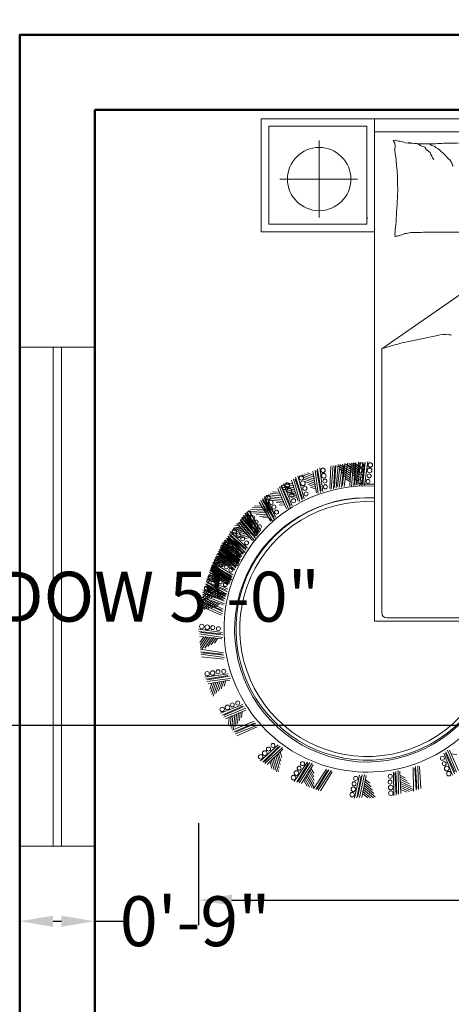
# Model space of a CAD drawing. Units: inches. Extents: x -59 to 502, y -260 to 136.
# Tile 3 of 8: x 25 to 77, y -53 to 66. Entities that reach past the tile are written whole.
import ezdxf

# ---------------------------------------------------------------- set-up
doc = ezdxf.new("R2010")
doc.units = ezdxf.units.IN
doc.header["$MEASUREMENT"] = 0
for name, color, linetype, lineweight in [('A-ANNO-DIMS', 2, 'Continuous', 18), ('Beds', 122, 'Continuous', 18), ('Outer Wall', 10, 'Continuous', 50), ('Windows', 150, 'Continuous', 18)]:
    doc.layers.add(name, color=color, linetype=linetype, lineweight=lineweight)
doc.styles.add('DIM_FONT', font='SIMPLEX.shx', dxfattribs={"width": 0.8})
doc.styles.get("Standard").update_dxf_attribs({"font": 'arial.ttf'})
doc.dimstyles.get("Standard").update_dxf_attribs({"dimtxt": 6, "dimasz": 4, "dimexe": 3, "dimexo": 3, "dimgap": 0.09, "dimtad": 0, "dimtih": 1, "dimtoh": 1, "dimdec": 1, "dimzin": 0, "dimdsep": 46, "dimlunit": 3, "dimtxsty": 'Standard', "dimcen": 0.09, "dimadec": 0, "dimazin": 0, "dimtfac": 1, "dimtdec": 1, "dimtofl": 0, "dimtmove": 0, "dimatfit": 3, "dimfxl": 1, "dimtolj": 1, "dimtzin": 0, "dimarcsym": 0})

# ---------------------------------------------------------------- blocks, each defined once
blk = doc.blocks.new('*D6')
at = {"layer": 'A-ANNO-DIMS', "color": 0, "lineweight": -2, "transparency": 16777216}
for p, q in [((22.46, 63.92), (-2.69, 63.92)), ((0.31, 59.92), (0.31, -58.98)), ((0.31, -184.08), (0.31, -65.18)), ((22.46, -188.08), (-2.69, -188.08))]:
    blk.add_line(p, q, dxfattribs=at)
at = {"layer": 'A-ANNO-DIMS', "color": 0, "transparency": 16777216}
for points in [[(-0.35, 59.92), (0.98, 59.92), (0.31, 63.92)], [(-0.35, -184.08), (0.98, -184.08), (0.31, -188.08)]]:
    blk.add_solid(points, dxfattribs=at)
at = {"layer": 'Defpoints', "color": 0, "transparency": 16777216}
for p in [(25.46, 63.92), (0.31, -188.08), (25.46, -188.08)]:
    blk.add_point(p, dxfattribs=at)
at = {"layer": 'A-ANNO-DIMS', "color": 0, "transparency": 16777216, "insert": (0.31, -62.08), "char_height": 6, "attachment_point": 5}
blk.add_mtext("\\A1;21'", dxfattribs=at)
blk = doc.blocks.new('*D7')
at = {"layer": 'A-ANNO-DIMS', "color": 0, "lineweight": -2, "transparency": 16777216}
for p, q in [((25.46, 66.92), (25.46, 89.09)), ((421.46, 66.92), (421.46, 89.09)), ((29.46, 86.09), (218.28, 86.09)), ((417.46, 86.09), (228.64, 86.09))]:
    blk.add_line(p, q, dxfattribs=at)
at = {"layer": 'A-ANNO-DIMS', "color": 0, "transparency": 16777216}
for points in [[(29.46, 86.75), (29.46, 85.42), (25.46, 86.09)], [(417.46, 86.75), (417.46, 85.42), (421.46, 86.09)]]:
    blk.add_solid(points, dxfattribs=at)
at = {"layer": 'Defpoints', "color": 0, "transparency": 16777216}
for p in [(421.46, 86.09), (25.46, 63.92), (421.46, 63.92)]:
    blk.add_point(p, dxfattribs=at)
at = {"layer": 'A-ANNO-DIMS', "color": 0, "transparency": 16777216, "insert": (223.46, 86.09), "char_height": 6, "attachment_point": 5}
blk.add_mtext("\\A1;33'", dxfattribs=at)
blk = doc.blocks.new('Window 1')
for p, q in [((840.32, 208.78), (900.32, 208.78)), ((840.32, 199.78), (840.32, 208.78)), ((900.32, 208.78), (900.32, 199.78)), ((840.32, 204.78), (900.32, 204.78)), ((900.32, 203.78), (840.32, 203.78)), ((900.32, 199.78), (840.32, 199.78))]:
    blk.add_line(p, q)
blk = doc.blocks.new('A$C187B6359')
for p, q in [((0.2493, 2.7052), (0.2493, 2.2552)), ((0.6993, 2.7052), (0.2493, 2.7052)), ((0.6993, 2.2552), (0.6993, 2.7052)), ((0.6999, 2.7053), (0.6999, 0.7053)), ((2.1999, 2.7053), (0.6999, 2.7053)), ((0.2793, 2.6752), (0.2793, 2.2852)), ((0.6693, 2.6752), (0.2793, 2.6752)), ((0.6693, 2.2852), (0.6693, 2.6752)), ((2.1999, 2.653), (0.6999, 2.653)), ((0.4797, 2.6178), (0.4797, 2.3115)), ((0.3236, 2.4648), (0.6327, 2.4648)), ((0.2793, 2.2852), (0.6693, 2.2852)), ((0.6727, 2.3088), (0.6721, 2.3088)), ((0.2493, 2.2552), (0.6993, 2.2552)), ((1.3464, 2.2168), (0.7284, 1.7894)), ((0.7284, 0.7375), (0.7284, 1.7894)), ((0.5923, 1.3337), (0.5787, 1.2403)), ((0.6165, 1.3344), (0.6081, 1.2403)), ((0.6432, 1.3092), (0.6087, 1.3332)), ((0.642, 1.3186), (0.6195, 1.3342)), ((0.6262, 1.3367), (0.6215, 1.2486)), ((0.6358, 1.339), (0.6275, 1.2449)), ((0.6437, 1.3345), (0.6342, 1.2469)), ((0.6535, 1.3363), (0.6399, 1.2428)), ((0.6633, 1.3381), (0.6538, 1.2504)), ((0.6731, 1.3398), (0.6595, 1.2463)), ((0.4577, 1.2862), (0.4318, 1.2951)), ((0.455, 1.302), (0.4698, 1.215)), ((0.4639, 1.3064), (0.4764, 1.2128)), ((0.4706, 1.3041), (0.4854, 1.2171)), ((0.4729, 1.3107), (0.4877, 1.2238)), ((0.4818, 1.3151), (0.4943, 1.2215)), ((0.5264, 1.3215), (0.5217, 1.2334)), ((0.5361, 1.3238), (0.5277, 1.2297)), ((0.5421, 1.3201), (0.5374, 1.232)), ((0.5458, 1.3261), (0.5411, 1.238)), ((0.5555, 1.3284), (0.5471, 1.2343)), ((0.5629, 1.3285), (0.5533, 1.2408)), ((0.6047, 1.292), (0.5545, 1.3229)), ((0.5727, 1.3302), (0.5591, 1.2368)), ((0.6051, 1.3), (0.5613, 1.327)), ((0.6042, 1.284), (0.5618, 1.3102)), ((0.5785, 1.3262), (0.5689, 1.2385)), ((0.6049, 1.2753), (0.569, 1.2975)), ((0.6077, 1.3067), (0.5719, 1.3288)), ((0.5825, 1.332), (0.5729, 1.2443)), ((0.6059, 1.3161), (0.5826, 1.3304)), ((0.6394, 1.2947), (0.5911, 1.3283)), ((0.6385, 1.2867), (0.5976, 1.3152)), ((0.6403, 1.3027), (0.5981, 1.332)), ((0.6068, 1.3321), (0.6021, 1.244)), ((0.6387, 1.278), (0.6041, 1.3021)), ((0.6225, 1.3307), (0.6178, 1.2426)), ((0.6593, 1.3323), (0.6497, 1.2446)), ((0.3747, 1.251), (0.3478, 1.2562)), ((0.3698, 1.2663), (0.3965, 1.1822)), ((0.3781, 1.2719), (0.4034, 1.1809)), ((0.385, 1.2705), (0.4116, 1.1864)), ((0.3863, 1.2774), (0.413, 1.1934)), ((0.3946, 1.283), (0.4199, 1.192)), ((0.4617, 1.2625), (0.406, 1.2816)), ((0.4604, 1.2704), (0.4117, 1.2871)), ((0.4631, 1.2546), (0.4159, 1.2708)), ((0.4614, 1.2774), (0.4216, 1.2911)), ((0.4656, 1.2462), (0.4257, 1.2599)), ((0.6034, 1.268), (0.5762, 1.2848)), ((0.6035, 1.2597), (0.5834, 1.2721)), ((0.6368, 1.2708), (0.6105, 1.289)), ((0.6364, 1.2624), (0.617, 1.2759)), ((0.3214, 1.2178), (0.2942, 1.2201)), ((0.315, 1.2325), (0.3505, 1.1518)), ((0.3226, 1.2389), (0.3575, 1.1512)), ((0.3819, 1.2281), (0.3242, 1.2393)), ((0.3795, 1.2357), (0.3291, 1.2455)), ((0.3296, 1.2383), (0.3651, 1.1576)), ((0.3302, 1.2453), (0.3657, 1.1646)), ((0.3844, 1.2204), (0.3354, 1.23)), ((0.3378, 1.2518), (0.3728, 1.164)), ((0.3796, 1.2429), (0.3383, 1.2509)), ((0.388, 1.2125), (0.3466, 1.2206)), ((0.4657, 1.2388), (0.4355, 1.2491)), ((0.4677, 1.2306), (0.4454, 1.2383)), ((0.6999, 1.25), (0.641, 1.25)), ((0.2407, 1.1781), (0.2871, 1.1031)), ((0.2474, 1.1856), (0.2941, 1.1035)), ((0.248, 1.1868), (0.2836, 1.1061)), ((0.254, 1.193), (0.3004, 1.1179)), ((0.2544, 1.1859), (0.3008, 1.1109)), ((0.2556, 1.1933), (0.2906, 1.1055)), ((0.2607, 1.2004), (0.3074, 1.1183)), ((0.2626, 1.1927), (0.2982, 1.1119)), ((0.2632, 1.1997), (0.2988, 1.1189)), ((0.2708, 1.2061), (0.3058, 1.1184)), ((0.3311, 1.1958), (0.2725, 1.2008)), ((0.3279, 1.2031), (0.2767, 1.2075)), ((0.3344, 1.1885), (0.2846, 1.1927)), ((0.3272, 1.2103), (0.2853, 1.2138)), ((0.3389, 1.181), (0.2968, 1.1846)), ((0.3408, 1.1738), (0.309, 1.1765)), ((0.3892, 1.2052), (0.3578, 1.2113)), ((0.3923, 1.1974), (0.3691, 1.2019)), ((0.194, 1.1385), (0.2404, 1.0634)), ((0.2007, 1.1459), (0.2474, 1.0638)), ((0.2618, 1.144), (0.203, 1.1409)), ((0.2576, 1.1509), (0.2063, 1.1481)), ((0.2559, 1.1578), (0.2139, 1.1555)), ((0.266, 1.1372), (0.2162, 1.1345)), ((0.2492, 1.1645), (0.2218, 1.163)), ((0.3447, 1.1664), (0.3212, 1.1684)), ((0.1599, 1.0992), (0.2209, 1.0271)), ((0.1651, 1.1077), (0.2244, 1.0425)), ((0.1667, 1.1009), (0.2261, 1.0356)), ((0.1678, 1.1099), (0.2241, 1.042)), ((0.1703, 1.1162), (0.2313, 1.0441)), ((0.1733, 1.1182), (0.231, 1.0434)), ((0.1789, 1.1264), (0.2352, 1.0585)), ((0.1802, 1.1195), (0.2366, 1.0516)), ((0.1807, 1.1237), (0.2271, 1.0486)), ((0.1845, 1.1347), (0.2421, 1.0599)), ((0.1874, 1.1311), (0.2341, 1.049)), ((0.1944, 1.1315), (0.2408, 1.0564)), ((0.2715, 1.1305), (0.2294, 1.1282)), ((0.2744, 1.1236), (0.2425, 1.1218)), ((0.2793, 1.1168), (0.2557, 1.1155)), ((0.1817, 1.0611), (0.1245, 1.0471)), ((0.1261, 1.0612), (0.1943, 0.9959)), ((0.1763, 1.067), (0.1264, 1.0548)), ((0.1734, 1.0735), (0.1325, 1.0636)), ((0.1934, 1.0791), (0.1356, 1.0678)), ((0.1882, 1.0852), (0.1378, 1.0754)), ((0.1655, 1.0789), (0.1389, 1.0724)), ((0.1856, 1.0919), (0.1444, 1.0838)), ((0.1985, 1.0729), (0.1495, 1.0633)), ((0.178, 1.0976), (0.1512, 1.0923)), ((0.1547, 1.0907), (0.2141, 1.0255)), ((0.2049, 1.067), (0.1634, 1.0589)), ((0.2087, 1.0605), (0.1774, 1.0544)), ((0.1253, 1.0235), (0.0995, 1.0143)), ((0.1057, 1.0262), (0.1651, 0.9609)), ((0.1109, 1.0347), (0.1719, 0.9626)), ((0.1133, 1.0342), (0.1792, 0.9755)), ((0.1161, 1.0432), (0.1754, 0.9779)), ((0.1176, 1.0432), (0.1858, 0.9779)), ((0.1178, 1.0363), (0.1771, 0.9711)), ((0.1213, 1.0517), (0.1823, 0.9796)), ((0.1218, 1.0522), (0.1877, 0.9935)), ((0.1242, 1.0456), (0.1901, 0.9869)), ((0.1871, 1.0551), (0.1386, 1.0433)), ((0.1937, 1.0495), (0.1527, 1.0395)), ((0.1979, 1.0433), (0.1668, 1.0357)), ((0.2039, 1.0375), (0.181, 1.0319)), ((0.2145, 1.0545), (0.1913, 1.05)), ((0.0799, 0.9828), (0.1458, 0.9242)), ((0.0814, 0.983), (0.1561, 0.9253)), ((0.0835, 0.9891), (0.1533, 0.9352)), ((0.0842, 0.9918), (0.1524, 0.9266)), ((0.0847, 0.9924), (0.1563, 0.941)), ((0.0847, 0.9891), (0.1588, 0.9306)), ((0.0871, 0.9983), (0.1598, 0.938)), ((0.0877, 0.9861), (0.1594, 0.9347)), ((0.1433, 1.0075), (0.0879, 0.9877)), ((0.0879, 1.0018), (0.1627, 0.9441)), ((0.088, 0.9985), (0.1592, 0.9463)), ((0.1373, 1.0129), (0.0889, 0.9955)), ((0.0907, 1.0076), (0.1605, 0.9537)), ((0.091, 0.9921), (0.1622, 0.94)), ((0.0914, 1.0078), (0.1656, 0.9493)), ((0.0935, 1.0012), (0.1634, 0.9473)), ((0.1337, 1.0191), (0.0941, 1.0049)), ((0.0943, 1.0169), (0.167, 0.9566)), ((0.1493, 1.0022), (0.1023, 0.9854)), ((0.1564, 0.9973), (0.1167, 0.9831)), ((0.1612, 0.9915), (0.1312, 0.9808)), ((0.1678, 0.9864), (0.1456, 0.9784)), ((0.1107, 0.9503), (0.0577, 0.9247)), ((0.1042, 0.9549), (0.0579, 0.9326)), ((0.1136, 0.956), (0.0603, 0.931)), ((0.1071, 0.9608), (0.0606, 0.9389)), ((0.1152, 0.9646), (0.0614, 0.9409)), ((0.1089, 0.9695), (0.0618, 0.9488)), ((0.0999, 0.9607), (0.0621, 0.9424)), ((0.103, 0.9666), (0.0649, 0.9487)), ((0.1049, 0.9754), (0.0664, 0.9585)), ((0.0911, 0.9643), (0.0665, 0.9524)), ((0.0942, 0.9703), (0.0694, 0.9586)), ((0.0962, 0.9793), (0.0711, 0.9683)), ((0.0714, 0.9648), (0.1373, 0.9062)), ((0.1172, 0.9456), (0.0723, 0.9239)), ((0.1201, 0.9513), (0.0749, 0.9301)), ((0.0756, 0.9738), (0.1439, 0.9085)), ((0.1216, 0.9597), (0.0759, 0.9396)), ((0.0781, 0.9736), (0.1498, 0.9222)), ((0.0813, 0.9797), (0.1524, 0.9276)), ((0.0823, 0.9762), (0.1482, 0.9175)), ((0.1249, 0.9415), (0.0869, 0.9231)), ((0.1277, 0.9471), (0.0895, 0.9292)), ((0.1291, 0.9553), (0.0905, 0.9383)), ((0.133, 0.9418), (0.1041, 0.9282)), ((0.1343, 0.9499), (0.105, 0.937)), ((0.1412, 0.9452), (0.1196, 0.9357)), ((0.0634, 0.9017), (0.0401, 0.8873)), ((0.0461, 0.9067), (0.1173, 0.8546)), ((0.047, 0.9096), (0.1217, 0.8519)), ((0.0494, 0.9097), (0.1261, 0.8661)), ((0.0495, 0.9161), (0.1236, 0.8576)), ((0.0503, 0.919), (0.122, 0.8676)), ((0.0517, 0.9194), (0.1321, 0.8698)), ((0.0529, 0.9254), (0.124, 0.8733)), ((0.0533, 0.9127), (0.125, 0.8613)), ((0.0535, 0.9284), (0.1283, 0.8707)), ((0.054, 0.9291), (0.1307, 0.8855)), ((0.0559, 0.9191), (0.127, 0.8669)), ((0.0563, 0.9387), (0.1367, 0.8892)), ((0.0563, 0.9348), (0.1304, 0.8763)), ((0.0577, 0.9231), (0.1344, 0.8795)), ((0.1302, 0.9362), (0.1015, 0.9224)), ((0.1373, 0.9318), (0.116, 0.9216)), ((0.1401, 0.9374), (0.1187, 0.9273)), ((0.0301, 0.8628), (0.111, 0.8276)), ((0.0314, 0.8727), (0.1166, 0.8319)), ((0.0773, 0.8938), (0.0336, 0.8667)), ((0.0843, 0.8899), (0.0343, 0.8589)), ((0.0725, 0.8991), (0.0368, 0.877)), ((0.0437, 0.9002), (0.1154, 0.8488)), ((0.0913, 0.8859), (0.0489, 0.8596)), ((0.0993, 0.8826), (0.0635, 0.8604)), ((0.1052, 0.878), (0.0781, 0.8612)), ((0.1127, 0.8744), (0.0927, 0.8619)), ((0.0571, 0.8302), (0.0165, 0.7987)), ((0.0171, 0.8298), (0.1045, 0.7938)), ((0.0644, 0.827), (0.0179, 0.7909)), ((0.0517, 0.835), (0.0185, 0.8092)), ((0.0424, 0.8367), (0.0208, 0.8199)), ((0.023, 0.8331), (0.0997, 0.7895)), ((0.0252, 0.8428), (0.1056, 0.7932)), ((0.0275, 0.8525), (0.1042, 0.8089)), ((0.0277, 0.8431), (0.1085, 0.8078)), ((0.0289, 0.8529), (0.1141, 0.8121)), ((0.0298, 0.8621), (0.1102, 0.8126)), ((0.0312, 0.8465), (0.1079, 0.8029)), ((0.0718, 0.8238), (0.0324, 0.7932)), ((0.0345, 0.8573), (0.1153, 0.822)), ((0.0452, 0.7888), (0.0064, 0.7551)), ((0.0396, 0.7933), (0.0079, 0.7657)), ((0.0527, 0.7861), (0.0083, 0.7474)), ((0.0301, 0.7944), (0.0095, 0.7765)), ((0.0131, 0.7937), (0.0983, 0.7529)), ((0.0151, 0.8), (0.0978, 0.7693)), ((0.0158, 0.8099), (0.1031, 0.774)), ((0.0165, 0.8199), (0.0992, 0.7892)), ((0.0211, 0.8145), (0.1038, 0.7839)), ((0.0801, 0.8214), (0.0468, 0.7955)), ((0.0865, 0.8174), (0.0612, 0.7978)), ((0.0943, 0.8146), (0.0757, 0.8001)), ((0.0094, 0.7641), (0.0902, 0.7289)), ((0.0106, 0.774), (0.0958, 0.7332)), ((0.0119, 0.7839), (0.0927, 0.7486)), ((0.0162, 0.7783), (0.0971, 0.743)), ((0.0602, 0.7833), (0.0226, 0.7505)), ((0.0687, 0.7813), (0.0369, 0.7536)), ((0.0752, 0.7777), (0.0512, 0.7567)), ((0.0832, 0.7753), (0.0654, 0.7598)), ((2.1541, 0.7175), (0.7484, 0.7175)), ((0, 0.6734), (0.0935, 0.6598)), ((0.6999, 0.7053), (2.1999, 0.7053)), ((0.0018, 0.6636), (0.0894, 0.654)), ((0.0035, 0.6538), (0.097, 0.6402)), ((0.0053, 0.644), (0.093, 0.6344)), ((0.0212, 0.6423), (0.0056, 0.6198)), ((0.0306, 0.6435), (0.0066, 0.609)), ((0.0075, 0.6596), (0.0952, 0.65)), ((0.0372, 0.6405), (0.0078, 0.5983)), ((0.0451, 0.6396), (0.0115, 0.5913)), ((0.0531, 0.6388), (0.0246, 0.5978)), ((0.0618, 0.639), (0.0377, 0.6043)), ((0.069, 0.637), (0.0508, 0.6108)), ((0.0774, 0.6367), (0.0639, 0.6173)), ((0.0061, 0.5926), (0.0995, 0.579)), ((0.0078, 0.5828), (0.0955, 0.5732)), ((0.0096, 0.573), (0.1031, 0.5594)), ((0.0113, 0.5632), (0.099, 0.5536)), ((0.0136, 0.5788), (0.1013, 0.5692)), ((0.0247, 0.4821), (0.1183, 0.4946)), ((0.0291, 0.4731), (0.116, 0.4879)), ((0.0334, 0.4642), (0.1271, 0.4767)), ((0.0357, 0.4708), (0.1227, 0.4857)), ((0.0378, 0.4552), (0.1248, 0.47)), ((0.0536, 0.4579), (0.0448, 0.4321)), ((0.0624, 0.4617), (0.0487, 0.4219)), ((0.0694, 0.4606), (0.0528, 0.412)), ((0.0773, 0.462), (0.0582, 0.4063)), ((0.0853, 0.4633), (0.0691, 0.4161)), ((0.0936, 0.4659), (0.0799, 0.426)), ((0.1011, 0.466), (0.0907, 0.4358)), ((0.1092, 0.468), (0.1015, 0.4456)), ((0.0881, 0.3381), (0.1758, 0.373)), ((0.0945, 0.3304), (0.1752, 0.366)), ((0.1009, 0.3228), (0.1886, 0.3578)), ((0.1015, 0.3299), (0.1822, 0.3654)), ((0.1073, 0.3152), (0.188, 0.3508)), ((0.122, 0.3217), (0.1197, 0.2944)), ((0.1296, 0.3275), (0.126, 0.2856)), ((0.1367, 0.3282), (0.1323, 0.2769)), ((0.144, 0.3314), (0.139, 0.2727)), ((0.1514, 0.3346), (0.1471, 0.2849)), ((0.1588, 0.3391), (0.1552, 0.2971)), ((0.166, 0.3411), (0.1633, 0.3093)), ((0.1734, 0.345), (0.1714, 0.3214)), ((0.1337, 0.2711), (0.2215, 0.3061)), ((0.1401, 0.2635), (0.2209, 0.299)), ((0.1466, 0.2559), (0.2343, 0.2908)), ((0.1472, 0.2629), (0.2279, 0.2985)), ((0.153, 0.2483), (0.2337, 0.2838)), ((0.2468, 0.148), (0.3166, 0.2116)), ((0.2555, 0.1431), (0.3185, 0.2048)), ((0.2623, 0.145), (0.3253, 0.2068)), ((0.2642, 0.1382), (0.334, 0.2019)), ((0.2729, 0.1334), (0.3359, 0.1951)), ((0.3015, 0.1614), (0.3176, 0.1048)), ((0.3073, 0.1671), (0.3208, 0.1191)), ((0.3126, 0.1739), (0.3241, 0.1333)), ((0.3187, 0.1783), (0.3274, 0.1475)), ((0.3243, 0.1845), (0.3307, 0.1618)), ((1.0105, 0.0909), (0.9754, 0.1786)), ((1.0181, 0.0974), (0.9824, 0.178)), ((1.0187, 0.1044), (0.9829, 0.185)), ((1.0257, 0.1038), (0.9905, 0.1915)), ((1.0333, 0.1102), (0.9976, 0.1909)), ((1.0034, 0.1763), (1.027, 0.1743)), ((0.2843, 0.1446), (0.2918, 0.1183)), ((0.2894, 0.1527), (0.3008, 0.1122)), ((0.2958, 0.1558), (0.3098, 0.1064)), ((0.3809, 0.0657), (0.4331, 0.1445)), ((0.3906, 0.0631), (0.4366, 0.1384)), ((0.3967, 0.0666), (0.4427, 0.1419)), ((0.4002, 0.0605), (0.4524, 0.1393)), ((0.4098, 0.0579), (0.4559, 0.1332)), ((0.4472, 0.12), (0.4589, 0.0996)), ((0.8555, 0.0282), (0.8535, 0.1226)), ((0.8649, 0.0315), (0.8599, 0.1196)), ((0.8679, 0.0379), (0.8629, 0.1259)), ((0.8743, 0.0349), (0.8723, 0.1293)), ((0.8837, 0.0382), (0.8787, 0.1263)), ((0.4211, 0.0807), (0.442, 0.0442)), ((0.4265, 0.0853), (0.4522, 0.0407)), ((0.4307, 0.0921), (0.4601, 0.0411)), ((0.4349, 0.099), (0.4598, 0.0557)), ((0.4385, 0.1069), (0.4595, 0.0703)), ((0.4433, 0.1127), (0.4592, 0.085)), ((0.4566, 0.0367), (0.5088, 0.1155)), ((0.4662, 0.0341), (0.5123, 0.1094)), ((0.4723, 0.0377), (0.5184, 0.1129)), ((0.4759, 0.0315), (0.528, 0.1103)), ((0.4855, 0.029), (0.5315, 0.1042)), ((0.6197, 0), (0.6408, 0.0921)), ((0.6296, 0.001), (0.6463, 0.0876)), ((0.6341, 0.0064), (0.6507, 0.093)), ((0.6396, 0.0019), (0.6606, 0.094)), ((0.6495, 0.0029), (0.6661, 0.0895)), ((0.7768, 0.0089), (0.7748, 0.1033)), ((0.7862, 0.0122), (0.7812, 0.1003)), ((0.7892, 0.0186), (0.7842, 0.1066)), ((0.7956, 0.0156), (0.7936, 0.11)), ((0.805, 0.0189), (0.7999, 0.107)), ((0.8003, 0.0912), (0.8216, 0.0811)), ((0.8013, 0.083), (0.8302, 0.0693)), ((0.4182, 0.0716), (0.4318, 0.0479)), ((0.657, 0.0423), (0.7025, 0.0049)), ((0.6585, 0.0501), (0.697, 0.0184)), ((0.659, 0.0588), (0.6916, 0.032)), ((0.6615, 0.0659), (0.6862, 0.0456)), ((0.6626, 0.0742), (0.6808, 0.0592)), ((0.8006, 0.0755), (0.8387, 0.0574)), ((0.8013, 0.044), (0.8393, 0.026)), ((0.8022, 0.0669), (0.8473, 0.0456)), ((0.8027, 0.0589), (0.8559, 0.0337)), ((0.8031, 0.0509), (0.8496, 0.0289)), ((0.652, 0.0281), (0.6845, 0.0014)), ((0.6525, 0.0186), (0.6736, 0.0013)), ((0.6555, 0.0344), (0.6952, 0.0017)), ((0.804, 0.0349), (0.8288, 0.0232))]:
    blk.add_line(p, q)
for centre, radius in [((0.4797, 2.4648), 0.126), ((0.6466, 1.3265), 0.00895), ((0.6832, 1.3267), 0.00895), ((0.495, 1.3053), 0.00895), ((0.6447, 1.3047), 0.00929), ((0.68, 1.3051), 0.00929), ((0.409, 1.2751), 0.00895), ((0.4149, 1.254), 0.00929), ((0.4979, 1.2836), 0.00929), ((0.5028, 1.2622), 0.00801), ((0.6414, 1.2602), 0.00801), ((0.6447, 1.2827), 0.00801), ((0.6743, 1.2609), 0.00801), ((0.6788, 1.2831), 0.00801), ((0.353, 1.2454), 0.00895), ((0.3611, 1.2251), 0.00929), ((0.4227, 1.2335), 0.00801), ((0.4275, 1.2112), 0.00801), ((0.5045, 1.2395), 0.00801), ((0.2766, 1.1962), 0.00895), ((0.2875, 1.1772), 0.00929), ((0.3711, 1.2055), 0.00801), ((0.3783, 1.184), 0.00801), ((0.2008, 1.1328), 0.00895), ((0.3, 1.1592), 0.00801), ((0.3101, 1.1388), 0.00801), ((0.1867, 1.1151), 0.00895), ((0.2008, 1.0984), 0.00929), ((0.2142, 1.1155), 0.00929), ((0.2291, 1.0994), 0.00801), ((0.1426, 1.0618), 0.00895), ((0.2165, 1.083), 0.00801), ((0.2301, 1.0648), 0.00801), ((0.2419, 1.0806), 0.00801), ((0.1107, 1.0186), 0.00895), ((0.1584, 1.0467), 0.00929), ((0.1756, 1.033), 0.00801), ((0.1911, 1.0163), 0.00801), ((0.1043, 1.0041), 0.00895), ((0.1078, 1.01), 0.00895), ((0.1216, 0.9908), 0.00929), ((0.1249, 0.9964), 0.00929), ((0.1276, 1.0047), 0.00929), ((0.1401, 0.979), 0.00801), ((0.1434, 0.9844), 0.00801), ((0.1457, 0.9922), 0.00801), ((0.1623, 0.9767), 0.00801), ((0.0722, 0.9428), 0.00895), ((0.1573, 0.964), 0.00801), ((0.1604, 0.9693), 0.00801), ((0.0909, 0.9313), 0.00929), ((0.1106, 0.9215), 0.00801), ((0.1292, 0.9085), 0.00801), ((0.0469, 0.8784), 0.00895), ((0.0666, 0.8689), 0.00929), ((0.0872, 0.8613), 0.00801), ((0.0323, 0.8363), 0.00895), ((0.0525, 0.828), 0.00929), ((0.0735, 0.8215), 0.00801), ((0.1071, 0.8503), 0.00801), ((0.094, 0.8117), 0.00801), ((0.0131, 0.6834), 0.00895), ((0.0347, 0.6803), 0.00929), ((0.0567, 0.6791), 0.00801), ((0.079, 0.6745), 0.00801), ((0.0777, 0.5031), 0.00801), ((0.1003, 0.5048), 0.00801), ((0.0345, 0.4953), 0.00895), ((0.0562, 0.4982), 0.00929), ((0.0944, 0.3533), 0.00895), ((0.1147, 0.3614), 0.00929), ((0.1343, 0.3714), 0.00801), ((0.1559, 0.3785), 0.00801), ((0.2784, 0.1954), 0.00801), ((0.296, 0.2097), 0.00801), ((0.2474, 0.1644), 0.00895), ((0.2635, 0.1792), 0.00929), ((0.9699, 0.1587), 0.00801), ((0.4, 0.1194), 0.00801), ((0.4136, 0.1376), 0.00801), ((0.9771, 0.1371), 0.00801), ((0.9871, 0.1175), 0.00929), ((0.3775, 0.0818), 0.00895), ((0.3895, 0.1001), 0.00929), ((0.625, 0.0788), 0.00801), ((0.7627, 0.0865), 0.00801), ((0.9953, 0.0972), 0.00895), ((0.6157, 0.0352), 0.00929), ((0.6186, 0.057), 0.00801), ((0.7618, 0.0638), 0.00801), ((0.7643, 0.042), 0.00929), ((0.6108, 0.0139), 0.00895), ((0.7648, 0.0201), 0.00895)]:
    blk.add_circle(centre, radius)
for centre, radius, start, end in [((0.7725, 2.6193), 0.00342, 291.7883, 340.436), ((0.7743, 2.6138), 0.00232, 340.436, 101.8931), ((0.7738, 2.6432), 0.0251, 274.3025, 291.7883), ((0.7804, 2.6146), 0.00428, 201.9904, 281.8931), ((0.7489, 2.5943), 0.0328, 338.579, 8.1335), ((0.7958, 2.6048), 0.0156, 158.579, 201.9904), ((0.7979, 2.6447), 0.0289, 239.3487, 274.3025), ((0.7951, 2.5622), 0.0539, 59.3487, 84.7408), ((0.7953, 1.7882), 0.8208, 84.7408, 88.0921), ((0.8611, 2.7059), 0.0992, 254.0648, 274.2159), ((0.9268, 2.6871), 0.0992, 233.9136, 254.0648), ((0.8855, 1.1114), 1.4943, 88.0921, 90.5757), ((0.9797, 2.6502), 0.0992, 216.1766, 233.9136), ((1.023, 2.8128), 0.234, 242.7604, 249.1397), ((1.0084, 1.7347), 0.8732, 90.5757, 94.8018), ((0.9873, 2.6543), 0.0768, 231.6114, 242.7604), ((1.0124, 2.8973), 0.2897, 267.4614, 274.8018), ((0.5389, 2.5307), 0.246, 8.1335, 12.1095), ((0.979, 2.592), 0.1983, 187.6809, 192.1095), ((1.6965, 2.6041), 0.9131, 183.3687, 187.6809), ((1.0154, 2.6015), 0.0992, 198.4397, 216.1766), ((1.2233, 2.8687), 0.3916, 226.1885, 231.6114), ((1.155, 2.7035), 0.2252, 219.0349, 226.1885), ((1.0425, 2.5644), 0.0493, 208.3168, 219.0349), ((1.1885, 2.6116), 0.2002, 203.0028, 208.3168), ((1.4701, 2.4627), 0.6787, 178.3669, 183.3687), ((2.1558, 2.35), 1.3652, 176.945, 178.3669), ((14.4012, 1.5554), 13.6356, 176.49514, 176.94504), ((1.1013, 2.2263), 0.3212, 170.0016, 176.4951), ((0.7623, 2.2404), 0.0193, 350.0016, 16.6978), ((0.7815, 2.2357), 0.00132, 16.6978, 97.1204), ((0.8072, 2.1521), 0.0875, 97.1204, 106.2212), ((0.8315, 2.1707), 0.0767, 106.2212, 117.2841), ((0.8, 2.2885), 0.0453, 282.869, 297.2841), ((0.8116, 2.3939), 0.1459, 273.574, 282.869), ((0.8383, 3.4157), 1.164, 270.2865, 273.574), ((1.0077, 7.9716), 5.7185, 269.0296, 270.2865), ((0.0604, 5.8083), 4.0646, 280.7276, 282.9255), ((0.9774, 1.9043), 0.0581, 262.2696, 280.7276), ((1.0326, 2.0362), 0.1942, 256.8096, 262.2696), ((0.2245, 3.554), 1.8351, 285.9352, 287.7364), ((0.6365, 2.4469), 0.6574, 282.9255, 285.9352), ((0.6715, 0.6736), 0.5699, 87.1307, 3.1127), ((0.6698, 0.67), 0.5261, 86.7143, 0.065), ((0.6715, 0.6736), 0.5225, 86.8806, 3.3918), ((0.6715, 0.6735), 0.5076, 86.694, 3.4914), ((0.7484, 0.7375), 0.02, 180, 270)]:
    blk.add_arc(centre, radius, start, end)
at = {"style": 'DIM_FONT', "text_generation_flag": 4, "width": 0.8, "flags": 9}
for tag in ['YSIZE', 'XSIZE']:
    blk.add_attdef(tag, (2.1999, 2.7053), '', height=0.0005, rotation=180, dxfattribs=at)
blk = doc.blocks.new('*D41')
at = {"layer": 'A-ANNO-DIMS', "color": 0, "lineweight": -2, "transparency": 16777216}
for p, q in [((22.46, 26.41), (13.46, 26.41)), ((16.46, 22.41), (16.46, -0.4)), ((16.46, -29.59), (16.46, -6.79)), ((22.46, -33.59), (13.46, -33.59))]:
    blk.add_line(p, q, dxfattribs=at)
at = {"layer": 'A-ANNO-DIMS', "color": 0, "transparency": 16777216}
for points in [[(15.79, 22.41), (17.13, 22.41), (16.46, 26.41)], [(15.79, -29.59), (17.13, -29.59), (16.46, -33.59)]]:
    blk.add_solid(points, dxfattribs=at)
at = {"layer": 'Defpoints', "color": 0, "transparency": 16777216}
for p in [(25.46, 26.41), (16.46, -33.59), (25.46, -33.59)]:
    blk.add_point(p, dxfattribs=at)
at = {"layer": 'A-ANNO-DIMS', "color": 0, "transparency": 16777216, "insert": (16.46, -3.59), "char_height": 6, "attachment_point": 5}
blk.add_mtext('\\A1;PRIMARY WINDOW 5\'-0"', dxfattribs=at)
blk = doc.blocks.new('*D42')
at = {"layer": 'A-ANNO-DIMS', "color": 0, "lineweight": -2, "transparency": 16777216}
for p, q in [((25.46, -36.59), (25.46, -45.59)), ((34.46, -36.59), (34.46, -45.59)), ((29.46, -42.59), (30.46, -42.59)), ((34.46, -42.59), (38.46, -42.59))]:
    blk.add_line(p, q, dxfattribs=at)
at = {"layer": 'A-ANNO-DIMS', "color": 0, "transparency": 16777216}
for points in [[(29.46, -41.93), (29.46, -43.26), (25.46, -42.59)], [(30.46, -41.93), (30.46, -43.26), (34.46, -42.59)]]:
    blk.add_solid(points, dxfattribs=at)
at = {"layer": 'Defpoints', "color": 0, "transparency": 16777216}
for p in [(25.46, -33.59), (34.46, -33.59), (34.46, -42.59)]:
    blk.add_point(p, dxfattribs=at)
at = {"layer": 'A-ANNO-DIMS', "color": 0, "transparency": 16777216, "insert": (46.52, -42.59), "char_height": 6, "attachment_point": 5}
blk.add_mtext('\\A1;0\'-9"', dxfattribs=at)
blk = doc.blocks.new('*D46')
at = {"layer": 'A-ANNO-DIMS', "color": 0, "lineweight": -2, "transparency": 16777216}
for p, q in [((46.92, -30.8), (46.92, -43.06)), ((126.95, -30.8), (126.95, -43.06)), ((50.92, -40.06), (78.85, -40.06)), ((122.95, -40.06), (95.01, -40.06))]:
    blk.add_line(p, q, dxfattribs=at)
at = {"layer": 'A-ANNO-DIMS', "color": 0, "transparency": 16777216}
for points in [[(50.92, -39.39), (50.92, -40.72), (46.92, -40.06)], [(122.95, -39.39), (122.95, -40.72), (126.95, -40.06)]]:
    blk.add_solid(points, dxfattribs=at)
at = {"layer": 'Defpoints', "color": 0, "transparency": 16777216}
for p in [(46.92, -27.8), (126.95, -27.8), (126.95, -40.06)]:
    blk.add_point(p, dxfattribs=at)
at = {"layer": 'A-ANNO-DIMS', "color": 0, "transparency": 16777216, "insert": (86.93, -40.06), "char_height": 6, "attachment_point": 5}
blk.add_mtext('\\A1;6\'-8"', dxfattribs=at)
blk = doc.blocks.new('*D57')
at = {"layer": 'A-ANNO-DIMS', "color": 0, "lineweight": -2, "transparency": 16777216}
for p, q in [((25.46, 66.92), (25.46, 130.25)), ((184.38, 66.92), (184.38, 130.25)), ((29.46, 127.25), (94.81, 127.25)), ((180.38, 127.25), (115.03, 127.25))]:
    blk.add_line(p, q, dxfattribs=at)
at = {"layer": 'A-ANNO-DIMS', "color": 0, "transparency": 16777216}
for points in [[(29.46, 127.91), (29.46, 126.58), (25.46, 127.25)], [(180.38, 127.91), (180.38, 126.58), (184.38, 127.25)]]:
    blk.add_solid(points, dxfattribs=at)
at = {"layer": 'Defpoints', "color": 0, "transparency": 16777216}
for p in [(184.38, 127.25), (25.46, 63.92), (184.38, 63.92)]:
    blk.add_point(p, dxfattribs=at)
at = {"layer": 'A-ANNO-DIMS', "color": 0, "transparency": 16777216, "insert": (104.92, 127.25), "char_height": 6, "attachment_point": 5}
blk.add_mtext('\\A1;13\'-3"', dxfattribs=at)
blk = doc.blocks.new('*D68')
at = {"layer": 'A-ANNO-DIMS', "color": 0, "lineweight": -2, "transparency": 16777216}
for p, q in [((163.46, -19.08), (-40.87, -19.08)), ((-37.87, -23.08), (-37.87, -37.42)), ((-37.87, -58.08), (-37.87, -43.73)), ((163.46, -62.08), (-40.87, -62.08))]:
    blk.add_line(p, q, dxfattribs=at)
at = {"layer": 'A-ANNO-DIMS', "color": 0, "transparency": 16777216}
for points in [[(-38.53, -23.08), (-37.2, -23.08), (-37.87, -19.08)], [(-38.53, -58.08), (-37.2, -58.08), (-37.87, -62.08)]]:
    blk.add_solid(points, dxfattribs=at)
at = {"layer": 'Defpoints', "color": 0, "transparency": 16777216}
for p in [(166.46, -19.08), (-37.87, -62.08), (166.46, -62.08)]:
    blk.add_point(p, dxfattribs=at)
at = {"layer": 'A-ANNO-DIMS', "color": 0, "transparency": 16777216, "insert": (-37.87, -40.58), "char_height": 6, "attachment_point": 5}
blk.add_mtext('\\A1;3\'-7"', dxfattribs=at)

msp = doc.modelspace()

# ---------------------------------------------------------------- linework, layer by layer
at = {"layer": 'Outer Wall'}
for p, q in [((34.46, 54.92), (166.46, 54.92)), ((34.46, -68.08), (34.46, 54.92))]:
    msp.add_line(p, q, dxfattribs=at)
msp.add_lwpolyline([(220.96, -188.08), (25.46, -188.08), (25.46, 63.92), (421.46, 63.92), (421.46, -188.08), (292.96, -188.08)], dxfattribs=at)

# ---------------------------------------------------------------- block references
at = {"layer": 'Beds', "xscale": 30.18588446845849, "yscale": 30.18588446845849, "zscale": 30.18588446845849}
msp.add_blockref('A$C187B6359', (46.92, -27.8), dxfattribs=at)
at = {"layer": 'Windows', "rotation": 270}
msp.add_blockref('Window 1', (-174.32, 866.73), dxfattribs=at)

# ---------------------------------------------------------------- dimensions: what is measured, and where the dimension line sits
at = {"layer": 'A-ANNO-DIMS'}
for base, p1, p2, override, picture, middle in [((184.38, 127.25), (25.46, 63.92), (184.38, 63.92), {"dimdec": 1, "dimlfac": 1, "dimrnd": 0, "dimzin": 1, "dimdsep": 46, "dimlunit": 4, "dimfrac": 2}, '*D57', (104.92, 127.25)), ((421.46, 86.09), (25.46, 63.92), (421.46, 63.92), {"dimclrd": 0, "dimclre": 0, "dimclrt": 0}, '*D7', (223.46, 86.09)), ((126.95, -40.06), (46.92, -27.8), (126.95, -27.8), {"dimdec": 1, "dimlfac": 1, "dimrnd": 0, "dimzin": 1, "dimdsep": 46, "dimlunit": 4, "dimfrac": 2}, '*D46', (86.93, -40.06)), ((34.46, -42.59), (25.46, -33.59), (34.46, -33.59), {"dimdec": 1, "dimlfac": 1, "dimrnd": 0, "dimzin": 1, "dimdsep": 46, "dimlunit": 4, "dimfrac": 2}, '*D42', (46.52, -42.59))]:
    dim = msp.add_linear_dim(base=base, p1=p1, p2=p2, dimstyle='Standard', override=override, dxfattribs=at)
    dim.commit()
    dim.dimension.update_dxf_attribs({"geometry": picture, "text_midpoint": middle})
for base, p1, p2, override, picture, middle in [((0.31, -188.08), (25.46, 63.92), (25.46, -188.08), {"dimclrd": 0, "dimclre": 0, "dimclrt": 0}, '*D6', (0.31, -62.08)), ((-37.87, -62.08), (166.46, -19.08), (166.46, -62.08), {"dimdec": 1, "dimlfac": 1, "dimrnd": 0, "dimzin": 1, "dimdsep": 46, "dimlunit": 4, "dimfrac": 2}, '*D68', (-37.87, -40.58))]:
    dim = msp.add_linear_dim(base=base, p1=p1, p2=p2, angle=90, dimstyle='Standard', override=override, dxfattribs=at)
    dim.commit()
    dim.dimension.update_dxf_attribs({"geometry": picture, "text_midpoint": middle})
dim = msp.add_linear_dim(base=(16.46, -33.59), p1=(25.46, 26.41), p2=(25.46, -33.59), angle=270, text='PRIMARY WINDOW <>', dimstyle='Standard', override={"dimdec": 1, "dimlfac": 1, "dimrnd": 0, "dimzin": 1, "dimdsep": 46, "dimlunit": 4, "dimfrac": 2}, dxfattribs=at)
dim.commit()
dim.dimension.update_dxf_attribs({"geometry": '*D41', "text_midpoint": (16.46, -3.59)})

doc.saveas('drawing.dxf')
